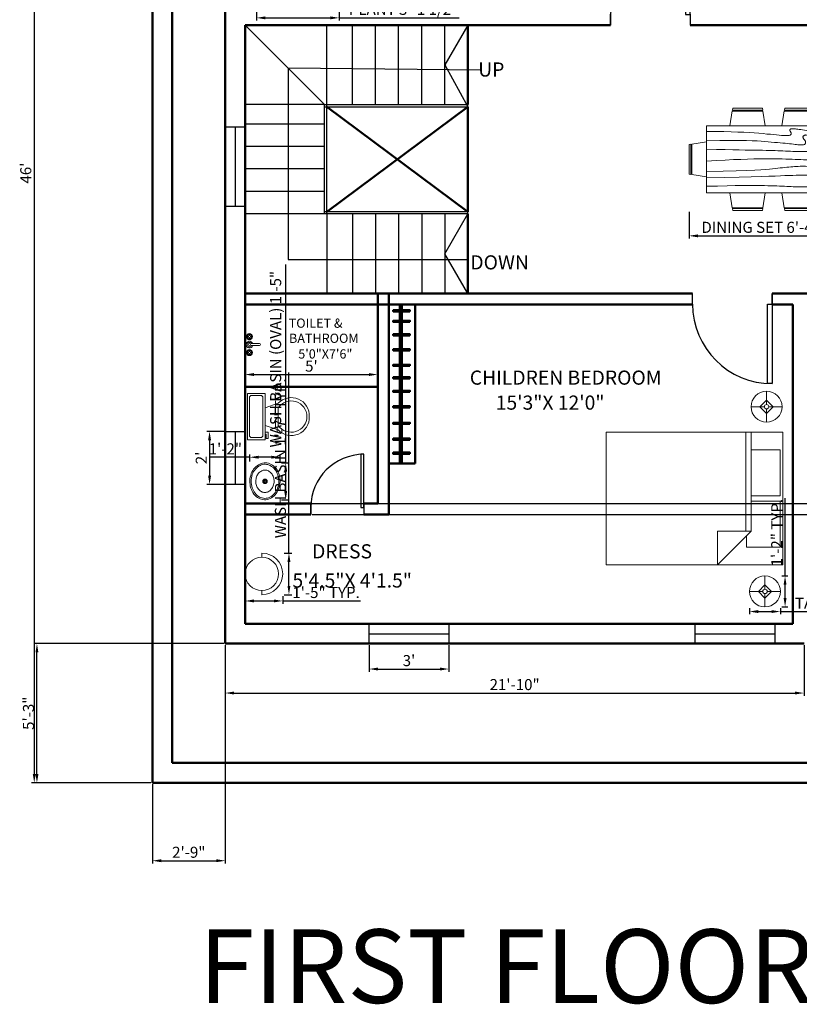
# Model space of a CAD drawing. Units: inches. Extents: x 116541 to 117938, y 135634 to 136328.
# Tile 5 of 9: x 117394 to 117747, y 135634 to 136080. Entities that reach past the tile are written whole.
import ezdxf

# ---------------------------------------------------------------- set-up
doc = ezdxf.new("R2010")
doc.units = ezdxf.units.IN
for name, color, linetype, lineweight in [('A-ANNO-DIMS', 2, 'Continuous', 18), ('A-ANNO-TEXT', 7, 'Continuous', 25), ('A-AREA-IDEN', 3, 'Continuous', 25), ('A-DOOR', 4, 'Continuous', 25), ('A-FLOR-FIXT', 9, 'Continuous', 18), ('A-FLOR-STRS', 2, 'Continuous', 25), ('A-FURN', 8, 'Continuous', 18), ('A-GLAZ', 1, 'Continuous', 25), ('A-WALL', 7, 'Continuous', 50)]:
    doc.layers.add(name, color=color, linetype=linetype, lineweight=lineweight)
doc.styles.get("Standard").update_dxf_attribs({"font": 'arial.ttf'})
doc.dimstyles.new('ISO-25', dxfattribs={"dimtxt": 5, "dimasz": 4, "dimexe": 1.25, "dimexo": 0.625, "dimtad": 1, "dimdec": 3, "dimlunit": 3, "dimtxsty": 'Standard', "dimcen": 2.5, "dimadec": 0, "dimazin": 0, "dimtfac": 1, "dimtdec": 3, "dimtmove": 0, "dimatfit": 3, "dimfxl": 1, "dimarcsym": 0})

# ---------------------------------------------------------------- blocks, each defined once
blk = doc.blocks.new('Sink - Oval top')
for p, q in [((-1, 0), (1, 0)), ((0, 1), (0, -1))]:
    blk.add_line(p, q)
for points in [[(-12.23, 0.39, 0.117634), (-11.46, -3.36, 0.104469), (-8.88, -6.8, 0.090016), (-5.08, -9.07, 0.08192), (-0.32, -10.02, 0.08192), (4.49, -9.38, 0.090016), (8.42, -7.36, 0.104469), (11.22, -4.09, 0.117634), (12.23, -0.39, 0.117634), (11.46, 3.36, 0.104469), (8.88, 6.8, 0.090016), (5.08, 9.07, 0.08192), (0.32, 10.02, 0.08192), (-4.49, 9.38, 0.090016), (-8.42, 7.36, 0.104469), (-11.22, 4.09, 0.117634)], [(-11.29, 0.16, 0.118622), (-10.52, -3.25, 0.104678), (-8.07, -6.36, 0.089562), (-4.54, -8.37, 0.081185), (-0.13, -9.15, 0.081185), (4.3, -8.49, 0.089562), (7.89, -6.58, 0.104678), (10.42, -3.55, 0.118622), (11.29, -0.16, 0.118622), (10.52, 3.25, 0.104678), (8.07, 6.36, 0.089562), (4.54, 8.37, 0.081185), (0.13, 9.15, 0.081185), (-4.3, 8.49, 0.089562), (-7.89, 6.58, 0.104678), (-10.42, 3.55, 0.118622)], [(-7.42, 0.08, 0.118283), (-6.91, -2.17, 0.104607), (-5.29, -4.21, 0.089718), (-2.97, -5.53, 0.081436), (-0.07, -6.04, 0.081436), (2.84, -5.59, 0.089718), (5.2, -4.33, 0.104607), (6.86, -2.32, 0.118283), (7.42, -0.08, 0.118283), (6.91, 2.17, 0.104607), (5.29, 4.21, 0.089718), (2.97, 5.53, 0.081436), (0.07, 6.04, 0.081436), (-2.84, 5.59, 0.089718), (-5.2, 4.33, 0.104607), (-6.86, 2.32, 0.118283)]]:
    blk.add_lwpolyline(points, format="xyb", close=True)
for radius in [1.5, 1]:
    blk.add_circle((0, 0), radius)
blk = doc.blocks.new('Dining Set - 36 x 72 in.')
for p, q in [((-22, 27.5), (-22.1562, 26.50042)), ((-5.8416, 26.5), (-22.1534, 26.5)), ((-22, 27.5), (-6, 27.5)), ((-5.8437, 26.49966), (-6, 27.5)), ((6, 27.5), (5.8438, 26.50042)), ((22.1584, 26.5), (5.8466, 26.5)), ((6, 27.5), (22, 27.5)), ((22.1563, 26.49966), (22, 27.5)), ((-22.2343, 26.00059), (-23.4847, 17.99762)), ((-22.2304, 26), (-5.7608, 26)), ((-4.5152, 17.99762), (-5.7655, 25.99926)), ((5.7657, 26.00059), (4.5153, 17.99762)), ((5.7696, 26), (22.2392, 26)), ((23.4848, 17.99762), (22.2345, 25.99926)), ((36, 18), (-36, 18)), ((-36, 18), (-36, -18)), ((36, -18), (36, 18)), ((-45.5, 8), (-44.5004, 8.15617)), ((-45.5, 8), (-45.5, -8)), ((-44.5, -8.15843), (-44.5, 8.15338)), ((-44.0006, 8.23428), (-35.9976, 9.48474)), ((-44, 8.23041), (-44, -8.23915)), ((44.0006, 8.23428), (35.9976, 9.48474)), ((44, 8.23041), (44, -8.23915)), ((44.5, -8.15843), (44.5, 8.15338)), ((45.5, 8), (44.5005, 8.15617)), ((45.5, 8), (45.5, -8)), ((-44.4997, -8.15631), (-45.5, -8)), ((-35.9976, -9.48476), (-43.9993, -8.2345)), ((35.9976, -9.48476), (43.9993, -8.2345)), ((44.4997, -8.15631), (45.5, -8)), ((-36, -18), (36, -18)), ((-22.2343, -26.0006), (-23.4847, -17.99762)), ((-4.5152, -17.99762), (-5.7655, -25.99928)), ((5.7657, -26.0006), (4.5153, -17.99762)), ((23.4848, -17.99762), (22.2345, -25.99928)), ((-22.2304, -26), (-5.7608, -26)), ((5.7696, -26), (22.2392, -26)), ((-22, -27.5), (-22.1562, -26.50044)), ((-5.8416, -26.5), (-22.1534, -26.5)), ((-22, -27.5), (-6, -27.5)), ((-5.8437, -26.49967), (-6, -27.5)), ((6, -27.5), (5.8438, -26.50044)), ((22.1584, -26.5), (5.8466, -26.5)), ((6, -27.5), (22, -27.5)), ((22.1563, -26.49967), (22, -27.5))]:
    blk.add_line(p, q)
for points in [[(-36, 15), (-31.1772, 14.97754), (-26.8079, 14.91406), (-22.8538, 14.81543), (-19.276, 14.6875), (-16.0362, 14.53613), (-13.0957, 14.36718), (-10.4159, 14.18652), (-7.9583, 14), (-5.6904, 13.81315), (-3.6035, 13.63021), (-1.6954, 13.45508), (0.0365, 13.29166), (1.5945, 13.14388), (2.9811, 13.01562), (4.1988, 12.9108), (5.25, 12.83333), (6.1393, 12.78613), (6.8802, 12.76823), (7.4883, 12.77767), (7.9792, 12.8125), (8.3685, 12.87077), (8.6719, 12.95052), (8.9049, 13.0498), (9.0833, 13.16666), (9.2205, 13.29899), (9.3216, 13.44401), (9.3895, 13.59879), (9.4271, 13.76041), (9.4373, 13.92594), (9.4232, 14.09245), (9.3875, 14.257), (9.3333, 14.41666), (9.2638, 14.56917), (9.1836, 14.71484), (9.0975, 14.85465), (9.0104, 14.98958), (8.9272, 15.1206), (8.8529, 15.2487), (8.7922, 15.37483), (8.75, 15.5), (8.7305, 15.62467), (8.7344, 15.74739), (8.7617, 15.86621), (8.8125, 15.97916), (8.8867, 16.08431), (8.9844, 16.17968), (9.1055, 16.26334), (9.25, 16.33333), (9.4189, 16.38802), (9.6172, 16.42708), (9.8506, 16.45052), (10.125, 16.45833), (10.4463, 16.45052), (10.8203, 16.42708), (11.2529, 16.38802), (11.75, 16.33333), (12.3184, 16.26318), (12.9694, 16.17838), (13.7151, 16.07991), (14.5677, 15.96875), (15.5395, 15.84586), (16.6426, 15.71224), (17.8893, 15.56884), (19.2917, 15.41666), (20.859, 15.25667), (22.5879, 15.08984), (24.4721, 14.91715), (26.5052, 14.73958), (28.6809, 14.5581), (30.9929, 14.3737), (33.4347, 14.18733), (36, 14)], [(-36, 10), (-28.9766, 10.14274), (-23.1725, 10.20442), (-18.4241, 10.19775), (-14.5677, 10.13541), (-11.4399, 10.03011), (-8.877, 9.89453), (-6.7154, 9.74137), (-4.7917, 9.58333), (-2.9698, 9.43082), (-1.2246, 9.28515), (0.4415, 9.14534), (2.026, 9.01041), (3.5266, 8.87939), (4.9408, 8.7513), (6.266, 8.62516), (7.5, 8.5), (8.6411, 8.37549), (9.6914, 8.2539), (10.6538, 8.13818), (11.5312, 8.03125), (12.3267, 7.93603), (13.043, 7.85547), (13.6831, 7.79248), (14.25, 7.75), (14.7471, 7.7303), (15.1797, 7.73307), (15.5537, 7.75732), (15.875, 7.80208), (16.1494, 7.86637), (16.3828, 7.94922), (16.5811, 8.04964), (16.75, 8.16666), (16.8944, 8.29915), (17.0143, 8.44531), (17.1089, 8.60319), (17.1771, 8.77083), (17.218, 8.94629), (17.2305, 9.1276), (17.2137, 9.31282), (17.1667, 9.5), (17.0895, 9.6875), (16.987, 9.875), (16.8649, 10.0625), (16.7292, 10.25), (16.5856, 10.4375), (16.4401, 10.625), (16.2985, 10.8125), (16.1667, 11), (16.05, 11.18733), (15.9518, 11.3737), (15.8752, 11.5581), (15.8229, 11.73958), (15.798, 11.91715), (15.8034, 12.08984), (15.842, 12.25667), (15.9167, 12.41666), (16.0295, 12.56836), (16.1784, 12.70833), (16.3605, 12.83268), (16.5729, 12.9375), (16.8127, 13.01888), (17.0768, 13.07291), (17.3625, 13.0957), (17.6667, 13.08333), (17.9894, 13.03312), (18.3418, 12.94726), (18.7382, 12.82918), (19.1927, 12.68229), (19.7195, 12.51001), (20.3327, 12.31575), (21.0465, 12.10294), (21.875, 11.875), (22.8357, 11.63354), (23.959, 11.37304), (25.2786, 11.08618), (26.8282, 10.76562), (28.6414, 10.40405), (30.752, 9.99414), (33.1936, 9.52856), (36, 9)], [(-36, 5.5), (-30.7157, 5.3348), (-26.069, 5.20963), (-21.9946, 5.11767), (-18.4271, 5.05208), (-15.3009, 5.00602), (-12.5508, 4.97265), (-10.1112, 4.94515), (-7.9167, 4.91666), (-5.909, 4.88167), (-4.0586, 4.83984), (-2.3429, 4.79215), (-0.7396, 4.73958), (0.7739, 4.6831), (2.22, 4.6237), (3.6213, 4.56233), (5, 4.5), (6.373, 4.43782), (7.7344, 4.3776), (9.0723, 4.32129), (10.375, 4.27083), (11.6309, 4.22819), (12.8281, 4.19531), (13.9551, 4.17415), (15, 4.16666), (15.954, 4.17448), (16.819, 4.19791), (17.6001, 4.23698), (18.3021, 4.29166), (18.9299, 4.36198), (19.4883, 4.44791), (19.9823, 4.54948), (20.4167, 4.66666), (20.7969, 4.79899), (21.1302, 4.94401), (21.4245, 5.09879), (21.6875, 5.26041), (21.9271, 5.42594), (22.1511, 5.59245), (22.3672, 5.757), (22.5834, 5.91666), (22.8065, 6.06868), (23.0404, 6.21093), (23.2879, 6.34147), (23.5521, 6.45833), (23.8358, 6.55957), (24.142, 6.64323), (24.4735, 6.70735), (24.8334, 6.75), (25.2235, 6.76969), (25.642, 6.76692), (26.0858, 6.74267), (26.5521, 6.69791), (27.0379, 6.63362), (27.5404, 6.55078), (28.0565, 6.45036), (28.5834, 6.33333), (29.1242, 6.19987), (29.7071, 6.04687), (30.3661, 5.87044), (31.1354, 5.66666), (32.0493, 5.43164), (33.142, 5.16146), (34.4475, 4.85221), (36, 4.5)], [(-36, -1), (-30.7915, -0.6591), (-26.0195, -0.38216), (-21.6519, -0.16284), (-17.6563, 0.00521), (-14.0005, 0.12833), (-10.6523, 0.21289), (-7.5796, 0.26522), (-4.75, 0.29166), (-2.134, 0.29793), (0.2878, 0.28711), (2.5317, 0.26163), (4.6146, 0.22396), (6.5529, 0.17651), (8.3633, 0.12174), (10.0623, 0.06209), (11.6667, 0), (13.1899, -0.06201), (14.6341, -0.1211), (15.9982, -0.17432), (17.2813, -0.21875), (18.4823, -0.25147), (19.6003, -0.26953), (20.6343, -0.27002), (21.5834, -0.25), (22.4481, -0.20768), (23.2357, -0.14584), (23.9549, -0.06836), (24.6146, 0.02083), (25.2235, 0.11784), (25.7904, 0.21875), (26.3241, 0.31966), (26.8334, 0.41666), (27.3265, 0.50618), (27.8099, 0.58593), (28.2894, 0.65397), (28.7709, 0.70833), (29.2601, 0.74707), (29.763, 0.76823), (30.2855, 0.76985), (30.8334, 0.75), (31.4088, 0.70784), (31.9994, 0.64713), (32.589, 0.57275), (33.1615, 0.48958), (33.7008, 0.4025), (34.1908, 0.3164), (34.6153, 0.23616), (34.9584, 0.16666), (35.2099, 0.11165), (35.3848, 0.07031), (35.504, 0.04069), (35.5886, 0.02083), (35.6594, 0.00879), (35.7377, 0.0026), (35.8442, 0.00032), (36, 0)], [(-36, -6.5), (-27.1843, -6.31267), (-20.084, -6.1263), (-14.469, -5.9419), (-10.1094, -5.76042), (-6.7752, -5.58285), (-4.2363, -5.41016), (-2.2629, -5.24333), (-0.625, -5.08334), (0.8708, -4.93099), (2.2715, -4.78646), (3.5872, -4.64974), (4.8281, -4.52084), (6.0046, -4.39974), (7.127, -4.28646), (8.2053, -4.18099), (9.25, -4.08334), (10.2705, -3.99382), (11.2734, -3.91407), (12.2647, -3.84603), (13.25, -3.79167), (14.2354, -3.75293), (15.2266, -3.73177), (16.2295, -3.73015), (17.25, -3.75), (18.2912, -3.79248), (19.3451, -3.85547), (20.4009, -3.93604), (21.4479, -4.03125), (22.4754, -4.13819), (23.4727, -4.25391), (24.4289, -4.37549), (25.3334, -4.5), (26.1785, -4.62492), (26.9694, -4.74935), (27.7145, -4.87281), (28.4219, -4.99479), (29.1, -5.11483), (29.7572, -5.23242), (30.4016, -5.34709), (31.0417, -5.45834), (31.6837, -5.56437), (32.3262, -5.65821), (32.9658, -5.73153), (33.599, -5.77604), (34.2224, -5.78345), (34.8327, -5.74545), (35.4264, -5.65373), (36, -5.5)], [(-36, -10), (-26.4022, -9.81299), (-18.4675, -9.62891), (-11.9839, -9.45069), (-6.7396, -9.28125), (-2.5226, -9.12354), (0.8789, -8.98047), (3.6769, -8.85498), (6.0833, -8.75), (8.2767, -8.66765), (10.3021, -8.60677), (12.1712, -8.56543), (13.8958, -8.54167), (15.4876, -8.53353), (16.9583, -8.53907), (18.3197, -8.55632), (19.5834, -8.58334), (20.7616, -8.61841), (21.8685, -8.66081), (22.9188, -8.71004), (23.9271, -8.76563), (24.9081, -8.82707), (25.8763, -8.89388), (26.8465, -8.96558), (27.8334, -9.04167), (28.8474, -9.12118), (29.8828, -9.20117), (30.93, -9.27824), (31.9792, -9.34896), (33.0205, -9.40991), (34.0443, -9.45768), (35.0407, -9.48885), (36, -9.5)], [(-36, -14.5), (-30.0881, -14.33513), (-25.0332, -14.21224), (-20.7312, -14.12647), (-17.0781, -14.07292), (-13.97, -14.04671), (-11.3027, -14.04297), (-8.9724, -14.05681), (-6.875, -14.08334), (-4.9224, -14.11833), (-3.0905, -14.16016), (-1.3709, -14.20785), (0.2448, -14.26042), (1.7647, -14.3169), (3.1973, -14.3763), (4.5507, -14.43767), (5.8333, -14.5), (7.0554, -14.5621), (8.235, -14.62175), (9.3922, -14.67652), (10.5469, -14.72396), (11.7192, -14.76164), (12.929, -14.78711), (14.1965, -14.79794), (15.5417, -14.79167), (16.9933, -14.76424), (18.6152, -14.70508), (20.4804, -14.60197), (22.6615, -14.44271), (25.2312, -14.21509), (28.2624, -13.9069), (31.8277, -13.50594), (36, -13)]]:
    blk.add_lwpolyline(points)
blk = doc.blocks.new('Bed - Queen')
for p, q in [((0, -80.00003), (0, 0)), ((0, 0), (59.99999, 0)), ((59.99999, 0), (59.99999, -80.00003)), ((7.99999, -1.2), (28.79998, -1.2)), ((7.99999, -14.4), (7.99999, -1.2)), ((28.79998, -1.2), (28.79998, -14.4)), ((31.19999, -1.2), (51.99999, -1.2)), ((31.19999, -14.4), (31.19999, -1.2)), ((51.99999, -1.2), (51.99999, -16.4)), ((0, -14.4), (44.8, -14.4)), ((44.8, -16.8), (0, -16.8)), ((59.99999, -29.6), (44.8, -14.4)), ((44.8, -14.4), (44.8, -29.6)), ((51.99999, -16.4), (46.79936, -16.4)), ((44.8, -29.6), (59.99999, -29.6)), ((59.99999, -80.00003), (0, -80.00003))]:
    blk.add_line(p, q)
blk = doc.blocks.new('*U45')
for p, q in [((9.5, -6), (9.5, -2)), ((-10, -8.5), (-8, -8.5)), ((-10, -9.5), (-10, -8.5)), ((-8, -8.5), (-8, -8)), ((-7, -8), (-7, -9.5)), ((-4, -8), (-6, -14)), ((4, -8), (6, -14)), ((-7, -9.5), (-10, -9.5)), ((4, -14), (-4, -14))]:
    blk.add_line(p, q)
blk.add_lwpolyline([(10.5, -8), (10.5, 0), (-10.5, 0), (-10.5, -8)], close=True)
for points in [[(-9.5, -2), (-9.5, -6)], [(8.5, -1), (-8.5, -1)], [(-8.5, -7), (8.5, -7)]]:
    blk.add_lwpolyline(points)
for centre, radius, start, end in [((-8.625, -1.875), 0.8839, 81.8699, 188.1301), ((8.625, -1.875), 0.8839, 351.8699, 98.1301), ((-8.625, -6.125), 0.8839, 171.869898, 278.1301), ((8.625, -6.125), 0.8839, 261.8699, 8.1301), ((-0.4772, -19.9188), 8.0953, 133.01722, 273.38), ((0.0374, -19.8731), 7.127, 124.50543, 269.7), ((-0.0373, -19.8731), 7.127, 270.3, 55.4946), ((0.4773, -19.9188), 8.0953, 266.62, 46.9828)]:
    blk.add_arc(centre, radius, start, end)
blk = doc.blocks.new('Faucet - Bathroom top')
for p, q in [((-4.107, 0.125), (-4.375, 0.125)), ((-3.75, 0.4788), (-3.75, 0.75)), ((-3.5, 0.482), (-3.5, 0.75)), ((-3.1461, 0.125), (-2.875, 0.125)), ((3.143, 0.125), (2.875, 0.125)), ((3.5, 0.4788), (3.5, 0.75)), ((3.75, 0.482), (3.75, 0.75)), ((4.1039, 0.125), (4.375, 0.125)), ((-4.1039, -0.125), (-4.375, -0.125)), ((-3.75, -0.4821), (-3.75, -0.75)), ((-3.5, -0.4789), (-3.5, -0.75)), ((-3.143, -0.125), (-2.875, -0.125)), ((-0.5, -0.8639), (-0.5, -4.5)), ((0.5, -4.5), (0.5, -0.8631)), ((3.1461, -0.125), (2.875, -0.125)), ((3.5, -0.4821), (3.5, -0.75)), ((3.75, -0.4789), (3.75, -0.75)), ((4.107, -0.125), (4.375, -0.125))]:
    blk.add_line(p, q)
for centre, radius in [((-3.625, 0), 1.375), ((-4.625, 0), 0.2795), ((-3.625, 0), 0.5), ((-3.625, 1), 0.2795), ((-2.625, 0), 0.2795), ((0, 0), 0.5), ((3.625, 0), 1.375), ((2.625, 0), 0.2795), ((3.625, 0), 0.5), ((3.625, 1), 0.2795), ((4.625, 0), 0.2795), ((-3.625, -1), 0.2795), ((3.625, -1), 0.2795)]:
    blk.add_circle(centre, radius)
for centre, radius, start, end in [((-3.625, 0), 1, 105.2407, 164.2093), ((-3.625, 0), 1, 16.44125, 74.07887), ((0, 0), 1.5, 289.6514, 250.3603), ((0, 0), 1, 300.3431, 239.7554), ((3.625, 0), 1, 106.12, 164.0884), ((3.625, 0), 1, 16.23422, 73.90469), ((-3.625, 0), 1, 196.2342, 253.9047), ((-3.625, 0), 1, 286.12, 344.0884), ((3.625, 0), 1, 196.4413, 254.0789), ((3.625, 0), 1, 285.2407, 344.2093), ((0, -4.5), 0.5, 180, 0)]:
    blk.add_arc(centre, radius, start, end)
blk = doc.blocks.new('Lamp - Table')
for p, q in [((0, 7), (0, 1)), ((-1, 0), (-7, 0)), ((0, 3), (-3, 0)), ((-3, 0), (0, -3)), ((3, 0), (0, 3)), ((0, -3), (3, 0)), ((1, 0), (7, 0)), ((0, -1), (0, -7))]:
    blk.add_line(p, q)
for radius in [7, 1]:
    blk.add_circle((0, 0), radius)
blk = doc.blocks.new('*U48')
for p, q in [((-750, 0), (-750, -100)), ((0, 0), (0, -100))]:
    blk.add_line(p, q)
blk.add_lwpolyline([(0, 0), (0, 750), (-43.75, 750), (-43.75, 0)], close=True)
blk.add_arc((0, 0), 750, 90, 180)
blk = doc.blocks.new('*U49')
for p, q in [((-750, 0), (-750, 100)), ((0, 0), (0, 100))]:
    blk.add_line(p, q)
blk.add_lwpolyline([(0, 0), (0, -750), (-43.75, -750), (-43.75, 0)], close=True)
blk.add_arc((0, 0), 750, 180, 270)
blk = doc.blocks.new('*D50')
at = {"layer": 'A-ANNO-DIMS', "color": 0, "lineweight": -2, "transparency": 16777216}
for p, q in [((117487.52, 135796.88), (117487.52, 135773.9)), ((117749.52, 135796.88), (117749.52, 135773.9)), ((117491.52, 135775.15), (117745.52, 135775.15))]:
    blk.add_line(p, q, dxfattribs=at)
at = {"layer": 'A-ANNO-DIMS', "color": 0, "transparency": 16777216}
for points in [[(117491.52, 135775.82), (117491.52, 135774.49), (117487.52, 135775.15)], [(117745.52, 135775.82), (117745.52, 135774.49), (117749.52, 135775.15)]]:
    blk.add_solid(points, dxfattribs=at)
at = {"layer": 'Defpoints', "color": 0, "transparency": 16777216}
for p in [(117487.52, 135797.5), (117749.52, 135797.5), (117749.52, 135775.15)]:
    blk.add_point(p, dxfattribs=at)
at = {"layer": 'A-ANNO-DIMS', "color": 0, "transparency": 16777216, "insert": (117618.52, 135778.33), "char_height": 5, "attachment_point": 5}
blk.add_mtext('21\'-10"', dxfattribs=at)
blk = doc.blocks.new('*D52')
at = {"layer": 'A-ANNO-DIMS', "color": 0, "lineweight": -2, "transparency": 16777216}
for p, q in [((117552.7, 135796.88), (117552.7, 135784.76)), ((117588.7, 135796.88), (117588.7, 135784.76)), ((117556.7, 135786.01), (117584.7, 135786.01))]:
    blk.add_line(p, q, dxfattribs=at)
at = {"layer": 'A-ANNO-DIMS', "color": 0, "transparency": 16777216}
for points in [[(117556.7, 135786.68), (117556.7, 135785.34), (117552.7, 135786.01)], [(117584.7, 135786.68), (117584.7, 135785.34), (117588.7, 135786.01)]]:
    blk.add_solid(points, dxfattribs=at)
at = {"layer": 'Defpoints', "color": 0, "transparency": 16777216}
for p in [(117552.7, 135797.5), (117588.7, 135797.5), (117588.7, 135786.01)]:
    blk.add_point(p, dxfattribs=at)
at = {"layer": 'A-ANNO-DIMS', "color": 0, "transparency": 16777216, "insert": (117570.7, 135789.19), "char_height": 5, "attachment_point": 5}
blk.add_mtext("3'", dxfattribs=at)
blk = doc.blocks.new('*D53')
at = {"layer": 'A-ANNO-DIMS', "color": 0, "lineweight": -2, "transparency": 16777216}
for p, q in [((117486.9, 135893.58), (117479.17, 135893.58)), ((117480.42, 135889.58), (117480.42, 135873.58)), ((117486.9, 135869.58), (117479.17, 135869.58))]:
    blk.add_line(p, q, dxfattribs=at)
at = {"layer": 'A-ANNO-DIMS', "color": 0, "transparency": 16777216}
for points in [[(117479.75, 135889.58), (117481.09, 135889.58), (117480.42, 135893.58)], [(117479.75, 135873.58), (117481.09, 135873.58), (117480.42, 135869.58)]]:
    blk.add_solid(points, dxfattribs=at)
at = {"layer": 'Defpoints', "color": 0, "transparency": 16777216}
for p in [(117487.52, 135893.58), (117480.42, 135869.58), (117487.52, 135869.58)]:
    blk.add_point(p, dxfattribs=at)
at = {"layer": 'A-ANNO-DIMS', "color": 0, "transparency": 16777216, "insert": (117477.29, 135881.58), "char_height": 5, "attachment_point": 5, "rotation": 90}
blk.add_mtext("2'", dxfattribs=at)
blk = doc.blocks.new('*D54')
at = {"layer": 'A-ANNO-DIMS', "color": 0, "lineweight": -2, "transparency": 16777216}
for p, q in [((117453.9, 136286.5), (117399.8, 136286.5)), ((117401.05, 136282.5), (117401.05, 135738.5)), ((117453.9, 135734.5), (117399.8, 135734.5))]:
    blk.add_line(p, q, dxfattribs=at)
at = {"layer": 'A-ANNO-DIMS', "color": 0, "transparency": 16777216}
for points in [[(117400.38, 136282.5), (117401.71, 136282.5), (117401.05, 136286.5)], [(117400.38, 135738.5), (117401.71, 135738.5), (117401.05, 135734.5)]]:
    blk.add_solid(points, dxfattribs=at)
at = {"layer": 'Defpoints', "color": 0, "transparency": 16777216}
for p in [(117454.52, 136286.5), (117401.05, 135734.5), (117454.52, 135734.5)]:
    blk.add_point(p, dxfattribs=at)
at = {"layer": 'A-ANNO-DIMS', "color": 0, "transparency": 16777216, "insert": (117397.87, 136010.5), "char_height": 5, "attachment_point": 5, "rotation": 90}
blk.add_mtext("46'", dxfattribs=at)
blk = doc.blocks.new('*D56')
at = {"layer": 'A-ANNO-DIMS', "color": 0, "lineweight": -2, "transparency": 16777216}
for p, q in [((117496.52, 135914.36), (117496.52, 135920.56)), ((117500.52, 135919.31), (117552.52, 135919.31)), ((117556.52, 135914.36), (117556.52, 135920.56))]:
    blk.add_line(p, q, dxfattribs=at)
at = {"layer": 'A-ANNO-DIMS', "color": 0, "transparency": 16777216}
for points in [[(117500.52, 135919.98), (117500.52, 135918.64), (117496.52, 135919.31)], [(117552.52, 135919.98), (117552.52, 135918.64), (117556.52, 135919.31)]]:
    blk.add_solid(points, dxfattribs=at)
at = {"layer": 'Defpoints', "color": 0, "transparency": 16777216}
for p in [(117556.52, 135919.31), (117496.52, 135913.74), (117556.52, 135913.74)]:
    blk.add_point(p, dxfattribs=at)
at = {"layer": 'A-ANNO-DIMS', "color": 0, "transparency": 16777216, "insert": (117526.52, 135922.48), "char_height": 5, "attachment_point": 5}
blk.add_mtext("5'", dxfattribs=at)
blk = doc.blocks.new('WASH-BASIN')
for p, q in [((7.56, 17), (7.56, 18.87)), ((7.56, 0), (7.56, 1.87))]:
    blk.add_line(p, q)
blk.add_circle((7.56, 9.43), 7.56)
blk.add_arc((7.56, 9.43), 9.43, 270, 90)
blk = doc.blocks.new('*D58')
at = {"layer": 'A-ANNO-DIMS', "color": 0, "lineweight": -2, "transparency": 16777216}
for p, q in [((117501.66, 136085.74), (117501.66, 136079.51)), ((117539.05, 136085.74), (117539.05, 136079.51)), ((117505.66, 136080.76), (117535.05, 136080.76)), ((117539.05, 136080.76), (117593.45, 136080.76))]:
    blk.add_line(p, q, dxfattribs=at)
at = {"layer": 'A-ANNO-DIMS', "color": 0, "transparency": 16777216}
for points in [[(117505.66, 136081.43), (117505.66, 136080.09), (117501.66, 136080.76)], [(117535.05, 136081.43), (117535.05, 136080.09), (117539.05, 136080.76)]]:
    blk.add_solid(points, dxfattribs=at)
at = {"layer": 'Defpoints', "color": 0, "transparency": 16777216}
for p in [(117501.66, 136086.37), (117539.05, 136086.37), (117539.05, 136080.76)]:
    blk.add_point(p, dxfattribs=at)
at = {"layer": 'A-ANNO-DIMS', "color": 0, "transparency": 16777216, "insert": (117568.25, 136083.97), "char_height": 5, "attachment_point": 5}
blk.add_mtext('PLANT 3\'-1 1/2"', dxfattribs=at)
blk = doc.blocks.new('*D64')
at = {"layer": 'A-ANNO-DIMS', "color": 0, "lineweight": -2, "transparency": 16777216}
for p, q in [((117514.89, 135879.38), (117514.89, 135969.15)), ((117513, 135879.38), (117516.14, 135879.38)), ((117514.89, 135866.6), (117514.89, 135875.38)), ((117513, 135862.6), (117516.14, 135862.6))]:
    blk.add_line(p, q, dxfattribs=at)
at = {"layer": 'A-ANNO-DIMS', "color": 0, "transparency": 16777216}
for points in [[(117514.22, 135875.38), (117515.55, 135875.38), (117514.89, 135879.38)], [(117514.22, 135866.6), (117515.55, 135866.6), (117514.89, 135862.6)]]:
    blk.add_solid(points, dxfattribs=at)
at = {"layer": 'Defpoints', "color": 0, "transparency": 16777216}
for p in [(117512.37, 135879.38), (117514.89, 135879.38), (117512.37, 135862.6)]:
    blk.add_point(p, dxfattribs=at)
at = {"layer": 'A-ANNO-DIMS', "color": 0, "transparency": 16777216, "insert": (117510.98, 135926.26), "char_height": 5, "attachment_point": 5, "rotation": 90}
blk.add_mtext('WASH BASIN (OVAL) 1\'-5"', dxfattribs=at)
blk = doc.blocks.new('*D65')
at = {"layer": 'A-ANNO-DIMS', "color": 0, "lineweight": -2, "transparency": 16777216}
for p, q in [((117498.61, 135880), (117498.61, 135883.14)), ((117512.37, 135880), (117512.37, 135883.14)), ((117498.61, 135881.89), (117480.54, 135881.89)), ((117508.37, 135881.89), (117502.61, 135881.89))]:
    blk.add_line(p, q, dxfattribs=at)
at = {"layer": 'A-ANNO-DIMS', "color": 0, "transparency": 16777216}
for points in [[(117502.61, 135882.56), (117502.61, 135881.23), (117498.61, 135881.89)], [(117508.37, 135882.56), (117508.37, 135881.23), (117512.37, 135881.89)]]:
    blk.add_solid(points, dxfattribs=at)
at = {"layer": 'Defpoints', "color": 0, "transparency": 16777216}
for p in [(117498.61, 135881.89), (117498.61, 135879.38), (117512.37, 135879.38)]:
    blk.add_point(p, dxfattribs=at)
at = {"layer": 'A-ANNO-DIMS', "color": 0, "transparency": 16777216, "insert": (117487.57, 135885.03), "char_height": 5, "attachment_point": 5}
blk.add_mtext('1\'-2"', dxfattribs=at)
blk = doc.blocks.new('*D68')
at = {"layer": 'A-ANNO-DIMS', "color": 0, "lineweight": -2, "transparency": 16777216}
for p, q in [((117724.85, 135813.5), (117724.85, 135810.78)), ((117728.85, 135812.03), (117734.85, 135812.03)), ((117738.85, 135813.5), (117738.85, 135810.78)), ((117738.85, 135812.03), (117819.74, 135812.03))]:
    blk.add_line(p, q, dxfattribs=at)
at = {"layer": 'A-ANNO-DIMS', "color": 0, "transparency": 16777216}
for points in [[(117728.85, 135812.7), (117728.85, 135811.36), (117724.85, 135812.03)], [(117734.85, 135812.7), (117734.85, 135811.36), (117738.85, 135812.03)]]:
    blk.add_solid(points, dxfattribs=at)
at = {"layer": 'Defpoints', "color": 0, "transparency": 16777216}
for p in [(117724.85, 135814.13), (117738.85, 135814.13), (117738.85, 135812.03)]:
    blk.add_point(p, dxfattribs=at)
at = {"layer": 'A-ANNO-DIMS', "color": 0, "transparency": 16777216, "insert": (117781.3, 135815.17), "char_height": 5, "attachment_point": 5}
blk.add_mtext('TABLE LAMP 1\'-2" TYP.', dxfattribs=at)
blk = doc.blocks.new('*D69')
at = {"layer": 'A-ANNO-DIMS', "color": 0, "lineweight": -2, "transparency": 16777216}
for p, q in [((117740.95, 135828.13), (117740.95, 135863.39)), ((117739.48, 135828.13), (117742.2, 135828.13)), ((117740.95, 135818.13), (117740.95, 135824.13)), ((117739.48, 135814.13), (117742.2, 135814.13))]:
    blk.add_line(p, q, dxfattribs=at)
at = {"layer": 'A-ANNO-DIMS', "color": 0, "transparency": 16777216}
for points in [[(117740.29, 135824.13), (117741.62, 135824.13), (117740.95, 135828.13)], [(117740.29, 135818.13), (117741.62, 135818.13), (117740.95, 135814.13)]]:
    blk.add_solid(points, dxfattribs=at)
at = {"layer": 'Defpoints', "color": 0, "transparency": 16777216}
for p in [(117738.85, 135828.13), (117740.95, 135828.13), (117738.85, 135814.13)]:
    blk.add_point(p, dxfattribs=at)
at = {"layer": 'A-ANNO-DIMS', "color": 0, "transparency": 16777216, "insert": (117737.82, 135847.76), "char_height": 5, "attachment_point": 5, "rotation": 90}
blk.add_mtext('1\'-2" TYP.', dxfattribs=at)
blk = doc.blocks.new('*D80')
at = {"layer": 'A-ANNO-DIMS', "color": 0, "lineweight": -2, "transparency": 16777216}
for p, q in [((117697.46, 135992.95), (117697.46, 135980.84)), ((117774.05, 135992.95), (117774.05, 135980.84)), ((117701.46, 135982.09), (117770.05, 135982.09))]:
    blk.add_line(p, q, dxfattribs=at)
at = {"layer": 'A-ANNO-DIMS', "color": 0, "transparency": 16777216}
for points in [[(117701.46, 135982.75), (117701.46, 135981.42), (117697.46, 135982.09)], [(117770.05, 135982.75), (117770.05, 135981.42), (117774.05, 135982.09)]]:
    blk.add_solid(points, dxfattribs=at)
at = {"layer": 'Defpoints', "color": 0, "transparency": 16777216}
for p in [(117697.46, 135993.58), (117774.05, 135993.58), (117774.05, 135982.09)]:
    blk.add_point(p, dxfattribs=at)
at = {"layer": 'A-ANNO-DIMS', "color": 0, "transparency": 16777216, "insert": (117735.75, 135985.3), "char_height": 5, "attachment_point": 5}
blk.add_mtext('DINING SET 6\'-4 1/2"', dxfattribs=at)
blk = doc.blocks.new('*D82')
at = {"layer": 'A-ANNO-DIMS', "color": 0, "lineweight": -2, "transparency": 16777216}
for p, q in [((117516.35, 135838.53), (117516.35, 135920.26)), ((117514.14, 135838.53), (117517.6, 135838.53)), ((117516.35, 135823.66), (117516.35, 135834.53)), ((117514.14, 135819.66), (117517.6, 135819.66))]:
    blk.add_line(p, q, dxfattribs=at)
at = {"layer": 'A-ANNO-DIMS', "color": 0, "transparency": 16777216}
for points in [[(117515.68, 135834.53), (117517.01, 135834.53), (117516.35, 135838.53)], [(117515.68, 135823.66), (117517.01, 135823.66), (117516.35, 135819.66)]]:
    blk.add_solid(points, dxfattribs=at)
at = {"layer": 'Defpoints', "color": 0, "transparency": 16777216}
for p in [(117513.52, 135838.53), (117516.35, 135838.53), (117513.52, 135819.66)]:
    blk.add_point(p, dxfattribs=at)
at = {"layer": 'A-ANNO-DIMS', "color": 0, "transparency": 16777216, "insert": (117513.14, 135881.39), "char_height": 5, "attachment_point": 5, "rotation": 90}
blk.add_mtext('WASH BASIN 1\'-7" TYP.', dxfattribs=at)
blk = doc.blocks.new('*D83')
at = {"layer": 'A-ANNO-DIMS', "color": 0, "lineweight": -2, "transparency": 16777216}
for p, q in [((117496.52, 135819.04), (117496.52, 135815.58)), ((117500.52, 135816.83), (117509.52, 135816.83)), ((117513.52, 135819.04), (117513.52, 135815.58)), ((117513.52, 135816.83), (117548.77, 135816.83))]:
    blk.add_line(p, q, dxfattribs=at)
at = {"layer": 'A-ANNO-DIMS', "color": 0, "transparency": 16777216}
for points in [[(117500.52, 135817.5), (117500.52, 135816.16), (117496.52, 135816.83)], [(117509.52, 135817.5), (117509.52, 135816.16), (117513.52, 135816.83)]]:
    blk.add_solid(points, dxfattribs=at)
at = {"layer": 'Defpoints', "color": 0, "transparency": 16777216}
for p in [(117496.52, 135819.66), (117513.52, 135819.66), (117513.52, 135816.83)]:
    blk.add_point(p, dxfattribs=at)
at = {"layer": 'A-ANNO-DIMS', "color": 0, "transparency": 16777216, "insert": (117533.15, 135820.01), "char_height": 5, "attachment_point": 5}
blk.add_mtext('1\'-5" TYP.', dxfattribs=at)
blk = doc.blocks.new('*D100')
at = {"layer": 'A-ANNO-DIMS', "color": 0, "lineweight": -2, "transparency": 16777216}
for p, q in [((117487.52, 135796.88), (117487.52, 135698)), ((117454.52, 135733.88), (117454.52, 135698)), ((117458.52, 135699.25), (117483.52, 135699.25))]:
    blk.add_line(p, q, dxfattribs=at)
at = {"layer": 'A-ANNO-DIMS', "color": 0, "transparency": 16777216}
for points in [[(117458.52, 135699.92), (117458.52, 135698.59), (117454.52, 135699.25)], [(117483.52, 135699.92), (117483.52, 135698.59), (117487.52, 135699.25)]]:
    blk.add_solid(points, dxfattribs=at)
at = {"layer": 'Defpoints', "color": 0, "transparency": 16777216}
for p in [(117487.52, 135797.5), (117454.52, 135734.5), (117487.52, 135699.25)]:
    blk.add_point(p, dxfattribs=at)
at = {"layer": 'A-ANNO-DIMS', "color": 0, "transparency": 16777216, "insert": (117471.02, 135702.43), "char_height": 5, "attachment_point": 5}
blk.add_mtext('2\'-9"', dxfattribs=at)
blk = doc.blocks.new('*D102')
at = {"layer": 'A-ANNO-DIMS', "color": 0, "lineweight": -2, "transparency": 16777216}
for p, q in [((117486.9, 135797.5), (117401.02, 135797.5)), ((117402.27, 135738.5), (117402.27, 135793.5)), ((117453.9, 135734.5), (117401.02, 135734.5))]:
    blk.add_line(p, q, dxfattribs=at)
at = {"layer": 'A-ANNO-DIMS', "color": 0, "transparency": 16777216}
for points in [[(117401.6, 135793.5), (117402.94, 135793.5), (117402.27, 135797.5)], [(117401.6, 135738.5), (117402.94, 135738.5), (117402.27, 135734.5)]]:
    blk.add_solid(points, dxfattribs=at)
at = {"layer": 'Defpoints', "color": 0, "transparency": 16777216}
for p in [(117402.27, 135797.5), (117487.52, 135797.5), (117454.52, 135734.5)]:
    blk.add_point(p, dxfattribs=at)
at = {"layer": 'A-ANNO-DIMS', "color": 0, "transparency": 16777216, "insert": (117399.09, 135766), "char_height": 5, "attachment_point": 5, "rotation": 90}
blk.add_mtext('5\'-3"', dxfattribs=at)
blk = doc.blocks.new('*D104')
at = {"layer": 'A-ANNO-DIMS', "color": 0, "lineweight": -2, "transparency": 16777216}
for p, q in [((117936.77, 135865), (117936.77, 135869)), ((117526.85, 135861), (117938.02, 135861)), ((117936.77, 135861), (117936.77, 135856)), ((117526.85, 135856), (117938.02, 135856)), ((117936.77, 135852), (117936.77, 135833.46))]:
    blk.add_line(p, q, dxfattribs=at)
at = {"layer": 'A-ANNO-DIMS', "color": 0, "transparency": 16777216}
for points in [[(117936.1, 135865), (117937.44, 135865), (117936.77, 135861)], [(117936.1, 135852), (117937.44, 135852), (117936.77, 135856)]]:
    blk.add_solid(points, dxfattribs=at)
at = {"layer": 'Defpoints', "color": 0, "transparency": 16777216}
for p in [(117526.22, 135861), (117526.22, 135856), (117936.77, 135856)]:
    blk.add_point(p, dxfattribs=at)
at = {"layer": 'A-ANNO-DIMS', "color": 0, "transparency": 16777216, "insert": (117933.59, 135840.73), "char_height": 5, "attachment_point": 5, "rotation": 90}
blk.add_mtext('0\'-5"', dxfattribs=at)

msp = doc.modelspace()

# ---------------------------------------------------------------- linework, layer by layer
at = {"layer": 'A-DOOR'}
for points in [[(117661.9632, 136077.5034), (117661.9632, 136082.5034)], [(117697.9632, 136082.5034), (117697.9632, 136077.5034)], [(117699.0567, 135951.0034), (117699.0567, 135956.0034)], [(117735.0567, 135956.0034), (117735.0567, 135951.0034)], [(117526.2247, 135856.0034), (117526.2247, 135861.0034)], [(117550.2247, 135861.0034), (117550.2247, 135856.0034)]]:
    msp.add_lwpolyline(points, dxfattribs=at)
at = {"layer": 'A-FLOR-STRS'}
for p, q in [((117496.5209, 135956.0034), (117496.5209, 136077.5034)), ((117496.5209, 136077.5034), (117597.3004, 136077.5034)), ((117532.5209, 136041.5034), (117496.5209, 136077.5034)), ((117533.5209, 136041.5034), (117533.5209, 136077.5034)), ((117545.1672, 136041.5034), (117545.1672, 136077.5034)), ((117555.5939, 136041.5034), (117555.5939, 136077.5034)), ((117566.0205, 136041.5034), (117566.0205, 136077.5034)), ((117576.4471, 136041.5034), (117576.4471, 136077.5034)), ((117586.8737, 136041.5034), (117586.8737, 136077.5034)), ((117597.3004, 136077.5034), (117586.8737, 136059.5034)), ((117597.3004, 136077.5034), (117597.3004, 136041.5034)), ((117603.4887, 136057.1528), (117515.9954, 136058.0288)), ((117515.9954, 136058.0288), (117515.9954, 135971.3461)), ((117586.8737, 136059.5034), (117597.3004, 136040.5034)), ((117532.5209, 136041.5034), (117496.5209, 136041.5034)), ((117532.5209, 136041.5034), (117597.3004, 136041.5034)), ((117532.5209, 135992.0034), (117532.5209, 136041.5034)), ((117532.5209, 136040.5034), (117597.3004, 136040.5034)), ((117533.5209, 135992.0034), (117533.5209, 136041.5034)), ((117597.3004, 136040.5034), (117597.3004, 136041.5034)), ((117532.5209, 136032.7092), (117496.5209, 136032.7092)), ((117532.5209, 136022.5327), (117496.5209, 136022.5327)), ((117532.5209, 136012.3563), (117496.5209, 136012.3563)), ((117532.5209, 136002.1799), (117496.5209, 136002.1799)), ((117532.5209, 135992.0034), (117496.5209, 135992.0034)), ((117597.3004, 135993.0034), (117532.5209, 135993.0034)), ((117597.3004, 135992.0034), (117532.5209, 135992.0034)), ((117533.5209, 135992.0034), (117533.5209, 135956.0034)), ((117545.1672, 135992.0034), (117545.1672, 135956.0034)), ((117555.5939, 135992.0034), (117555.5939, 135956.0034)), ((117566.0205, 135992.0034), (117566.0205, 135956.0034)), ((117576.4471, 135992.0034), (117576.4471, 135956.0034)), ((117586.8737, 135992.0034), (117586.8737, 135956.0034)), ((117586.8737, 135974.0034), (117597.3004, 135992.0034)), ((117597.3004, 135992.0034), (117597.3004, 135993.0034)), ((117597.3004, 135992.0034), (117597.3004, 135956.0034)), ((117597.3004, 135956.0034), (117586.8737, 135974.0034)), ((117515.9954, 135971.3461), (117597.3004, 135971.3461)), ((117597.3004, 135956.0034), (117496.5209, 135956.0034))]:
    msp.add_line(p, q, dxfattribs=at)
at = {"layer": 'A-GLAZ'}
for p, q in [((117492.0209, 136031.4134), (117492.0209, 135995.4134)), ((117492.0209, 135893.5835), (117492.0209, 135869.5835)), ((117552.7038, 135802.0034), (117588.7038, 135802.0034)), ((117700.2693, 135802.0034), (117736.2693, 135802.0034))]:
    msp.add_line(p, q, dxfattribs=at)
for points in [[(117487.5209, 136031.4134), (117496.5209, 136031.4134), (117496.5209, 135995.4134), (117487.5209, 135995.4134)], [(117487.5209, 135893.5835), (117496.5209, 135893.5835), (117496.5209, 135869.5835), (117487.5209, 135869.5835)], [(117552.7038, 135797.5034), (117552.7038, 135806.5034), (117588.7038, 135806.5034), (117588.7038, 135797.5034)], [(117700.2693, 135797.5034), (117700.2693, 135806.5034), (117736.2693, 135806.5034), (117736.2693, 135797.5034)]]:
    msp.add_lwpolyline(points, close=True, dxfattribs=at)
at = {"layer": 'A-WALL'}
for p, q in [((117454.5209, 136286.5034), (117454.5209, 135734.5034)), ((117463.5209, 136277.5034), (117463.5209, 135743.5034)), ((117487.5209, 136253.5034), (117487.5209, 135797.5034)), ((117496.5209, 136077.5034), (117496.5209, 135806.5034)), ((117661.9632, 136077.5034), (117496.5209, 136077.5034)), ((117597.3004, 136041.5034), (117597.3004, 136077.5034)), ((117835.5209, 136077.5034), (117697.9632, 136077.5034)), ((117597.3004, 135993.0034), (117533.5209, 136040.5034)), ((117533.5209, 135993.0034), (117597.3004, 136040.5034)), ((117597.3004, 135993.0034), (117597.3004, 136040.5034)), ((117597.3004, 135956.0034), (117597.3004, 135992.0034)), ((117496.5209, 135956.0034), (117699.0567, 135956.0034)), ((117556.5209, 135956.0034), (117556.5209, 135861.0034)), ((117561.5209, 135956.0034), (117561.5209, 135856.0034)), ((117735.0567, 135956.0034), (117757.1864, 135956.0034)), ((117496.5209, 135951.0034), (117699.0567, 135951.0034)), ((117561.5209, 135951.0034), (117573.5209, 135951.0034)), ((117566.5209, 135951.0034), (117566.5209, 135879.0034)), ((117567.5209, 135951.0034), (117567.5209, 135879.0034)), ((117573.5209, 135951.0034), (117573.5209, 135879.0034)), ((117735.0567, 135951.0034), (117744.5209, 135951.0034)), ((117735.0567, 135951.0034), (117744.5209, 135951.0034)), ((117744.5209, 135951.0034), (117744.5209, 135806.5034)), ((117496.5209, 135913.7394), (117556.5209, 135913.7394)), ((117573.5209, 135879.0034), (117561.5209, 135879.0034)), ((117496.5209, 135861.0034), (117526.2247, 135861.0034)), ((117550.2247, 135861.0034), (117556.5209, 135861.0034)), ((117496.5209, 135856.0034), (117526.2247, 135856.0034)), ((117550.2247, 135856.0034), (117561.5209, 135856.0034)), ((117496.5209, 135806.5034), (117744.5209, 135806.5034)), ((117487.5209, 135797.5034), (117749.5209, 135797.5034)), ((117496.5209, 135797.5034), (117709.5209, 135797.5034)), ((117463.5209, 135743.5034), (117698.4977, 135743.5034)), ((117698.4977, 135743.5034), (117892.5209, 135743.5034)), ((117454.5209, 135734.5034), (117871.5209, 135734.5034))]:
    msp.add_line(p, q, dxfattribs=at)
for points in [[(117571.0826, 135947.8727), (117563.5528, 135947.8727), (117563.5528, 135948.423), (117571.0826, 135948.423)], [(117571.0826, 135943.1424), (117563.5528, 135943.1424), (117563.5528, 135943.6927), (117571.0826, 135943.6927)], [(117571.0826, 135937.0149), (117563.5528, 135937.0149), (117563.5528, 135937.5652), (117571.0826, 135937.5652)], [(117571.0826, 135930.2311), (117563.5528, 135930.2311), (117563.5528, 135930.7814), (117571.0826, 135930.7814)], [(117571.0826, 135923.2286), (117563.5528, 135923.2286), (117563.5528, 135923.7789), (117571.0826, 135923.7789)], [(117571.0826, 135917.5389), (117563.5528, 135917.5389), (117563.5528, 135918.0892), (117571.0826, 135918.0892)], [(117571.0826, 135911.4116), (117563.5528, 135911.4116), (117563.5528, 135911.9619), (117571.0826, 135911.9619)], [(117571.0826, 135904.4091), (117563.5528, 135904.4091), (117563.5528, 135904.9594), (117571.0826, 135904.9594)], [(117571.0826, 135896.9688), (117563.5528, 135896.9688), (117563.5528, 135897.5191), (117571.0826, 135897.5191)], [(117571.0826, 135889.7472), (117563.5528, 135889.7472), (117563.5528, 135890.2975), (117571.0826, 135890.2975)], [(117571.0826, 135883.401), (117563.5528, 135883.401), (117563.5528, 135883.9513), (117571.0826, 135883.9513)]]:
    msp.add_lwpolyline(points, close=True, dxfattribs=at)

# ---------------------------------------------------------------- block references
at = {"layer": 'A-DOOR'}
for name, p, xscale, yscale, zscale in [('*U48', (117697.9632, 136082.3034), 0.0480000000000013, 0.0480000000000013, 0.0480000000000013), ('*U49', (117735.0567, 135951.2034), 0.0480000000000013, 0.0480000000000013, 0.0480000000000013), ('*U48', (117550.2247, 135859.2034), 0.0320000000000009, 0.0320000000000009, 0.0320000000000009)]:
    msp.add_blockref(name, p, dxfattribs=dict(at, xscale=xscale, yscale=yscale, zscale=zscale))
at = {"layer": 'A-FLOR-FIXT', "rotation": 89.99999999999999}
msp.add_blockref('Faucet - Bathroom top', (117498.4848, 135932.8922), dxfattribs=at)
at = {"layer": 'A-FLOR-FIXT', "xscale": 0.683347719268136, "yscale": 0.683347719268136, "zscale": 0.683347719268136, "rotation": 90}
msp.add_blockref('Sink - Oval top', (117505.4904, 135870.9898), dxfattribs=at)
at = {"layer": 'A-FLOR-FIXT'}
msp.add_blockref('WASH-BASIN', (117496.521, 135819.66), dxfattribs=at)
at = {"layer": 'A-FURN', "xscale": 0.8416470728042412, "yscale": 0.8416470728042412, "zscale": 0.8416470728042412}
msp.add_blockref('Dining Set - 36 x 72 in.', (117735.7537, 136016.7204), dxfattribs=at)
at = {"layer": 'A-FURN'}
for name, p, rotation in [('*U45', (117497.5209, 135900.2939), 90), ('Bed - Queen', (117739.9362, 135893.224), 270)]:
    msp.add_blockref(name, p, dxfattribs=dict(at, rotation=rotation))
for p in [(117732.5647, 135904.7479), (117731.853, 135821.1291)]:
    msp.add_blockref('Lamp - Table', p, dxfattribs=at)

# ---------------------------------------------------------------- texts
at = {"layer": 'A-ANNO-TEXT'}
for s, height, p in [('UP', 6.40837, (117602.0334, 136054.1847)), ('DOWN', 6.40837, (117598.477, 135966.8827)), ('FIRST FLOOR PLAN', 33.340721, (117475.5022, 135634.8462))]:
    msp.add_text(s, height=height, dxfattribs=at).set_placement(p)
at = {"layer": 'A-AREA-IDEN'}
for s, height, p in [('TOILET &', 4.18062, (117516.244, 135940.4898)), ('BATHROOM', 4.18062, (117516.3924, 135933.6368)), ('5\'0"X7\'6"', 4.18062, (117520.5707, 135926.5554)), ('CHILDREN BEDROOM', 6.408368, (117598.2224, 135914.7164)), ('      15\'3"X 12\'0"', 6.408368, (117598.2224, 135903.4003)), ('DRESS', 6.40837, (117526.8308, 135836.0839)), ('5\'4.5"X 4\'1.5"', 6.408368, (117517.9469, 135822.9168))]:
    msp.add_text(s, height=height, dxfattribs=at).set_placement(p)

# ---------------------------------------------------------------- dimensions: what is measured, and where the dimension line sits
at = {"layer": 'A-ANNO-DIMS'}
for base, p1, p2, angle, override, picture, middle in [((117401.0451, 135734.5034), (117454.5209, 136286.5034), (117454.5209, 135734.5034), 90, {"dimclrd": 0, "dimclre": 0, "dimclrt": 0}, '*D54', (117397.8672, 136010.5034)), ((117480.4204, 135869.5835), (117487.5209, 135893.5835), (117487.5209, 135869.5835), 90, {"dimclrd": 0, "dimclre": 0, "dimclrt": 0}, '*D53', (117477.2852, 135881.5835)), ((117498.6103, 135881.8947), (117512.3706, 135879.3782), (117498.6103, 135879.3782), 180, {"dimdec": 1, "dimrnd": 0, "dimzin": 1, "dimlunit": 4, "dimfrac": 2}, '*D65', (117487.575, 135885.03)), ((117936.7709, 135856.0034), (117526.2247, 135861.0034), (117526.2247, 135856.0034), 90, {"dimdec": 1, "dimlfac": 1, "dimrnd": 0, "dimzin": 1, "dimdsep": 46, "dimlunit": 4, "dimfrac": 2}, '*D104', (117933.593, 135840.7328)), ((117402.2709, 135797.5034), (117454.5209, 135734.5034), (117487.5209, 135797.5034), 90, {"dimdec": 1, "dimlfac": 1, "dimrnd": 0, "dimzin": 1, "dimdsep": 46, "dimlunit": 4, "dimfrac": 2}, '*D102', (117399.0913, 135766.0034))]:
    dim = msp.add_linear_dim(base=base, p1=p1, p2=p2, angle=angle, dimstyle='ISO-25', override=override, dxfattribs=at)
    dim.commit()
    dim.dimension.update_dxf_attribs({"geometry": picture, "text_midpoint": middle})
for base, p1, p2, text, picture, middle in [((117539.048, 136080.7602), (117501.6552, 136086.3691), (117539.048, 136086.3691), 'PLANT <>', '*D58', (117568.2467, 136083.9722)), ((117774.0487, 135982.0866), (117697.4588, 135993.5751), (117774.0487, 135993.5751), 'DINING SET <>', '*D80', (117735.7537, 135985.2969)), ((117738.853, 135812.0291), (117724.853, 135814.1291), (117738.853, 135814.1291), 'TABLE LAMP <> TYP.', '*D68', (117781.2952, 135815.166)), ((117513.5171, 135816.8304), (117496.5209, 135819.6605), (117513.5171, 135819.6605), '<> TYP.', '*D83', (117533.1455, 135820.0083))]:
    dim = msp.add_linear_dim(base=base, p1=p1, p2=p2, text=text, dimstyle='ISO-25', override={"dimdec": 1, "dimrnd": 0, "dimzin": 1, "dimlunit": 4, "dimfrac": 2}, dxfattribs=at)
    dim.commit()
    dim.dimension.update_dxf_attribs({"geometry": picture, "text_midpoint": middle})
for base, p1, p2, text, picture, middle in [((117514.8871, 135879.3782), (117512.3706, 135862.6014), (117512.3706, 135879.3782), 'WASH BASIN (OVAL) <>', '*D64', (117510.9828, 135926.2645)), ((117516.3471, 135838.5272), (117513.5171, 135819.6605), (117513.5171, 135838.5272), 'WASH BASIN <> TYP.', '*D82', (117513.1369, 135881.3923)), ((117740.953, 135828.1291), (117738.853, 135814.1291), (117738.853, 135828.1291), '<> TYP.', '*D69', (117737.8161, 135847.7575))]:
    dim = msp.add_linear_dim(base=base, p1=p1, p2=p2, angle=90, text=text, dimstyle='ISO-25', override={"dimdec": 1, "dimrnd": 0, "dimzin": 1, "dimlunit": 4, "dimfrac": 2}, dxfattribs=at)
    dim.commit()
    dim.dimension.update_dxf_attribs({"geometry": picture, "text_midpoint": middle})
for base, p1, p2, override, picture, middle in [((117556.5209, 135919.3112), (117496.5209, 135913.7394), (117556.5209, 135913.7394), {"dimclrd": 0, "dimclre": 0, "dimclrt": 0}, '*D56', (117526.5209, 135922.4789)), ((117487.5209, 135699.2534), (117454.5209, 135734.5034), (117487.5209, 135797.5034), {"dimdec": 1, "dimlfac": 1, "dimrnd": 0, "dimzin": 1, "dimdsep": 46, "dimlunit": 4, "dimfrac": 2}, '*D100', (117471.0209, 135702.4313)), ((117749.5209, 135775.1534), (117487.5209, 135797.5034), (117749.5209, 135797.5034), {"dimclrd": 0, "dimclre": 0, "dimclrt": 0}, '*D50', (117618.5209, 135778.3313)), ((117588.7038, 135786.0112), (117552.7038, 135797.5034), (117588.7038, 135797.5034), {"dimclrd": 0, "dimclre": 0, "dimclrt": 0}, '*D52', (117570.7038, 135789.1907))]:
    dim = msp.add_linear_dim(base=base, p1=p1, p2=p2, dimstyle='ISO-25', override=override, dxfattribs=at)
    dim.commit()
    dim.dimension.update_dxf_attribs({"geometry": picture, "text_midpoint": middle})

doc.saveas('drawing.dxf')
